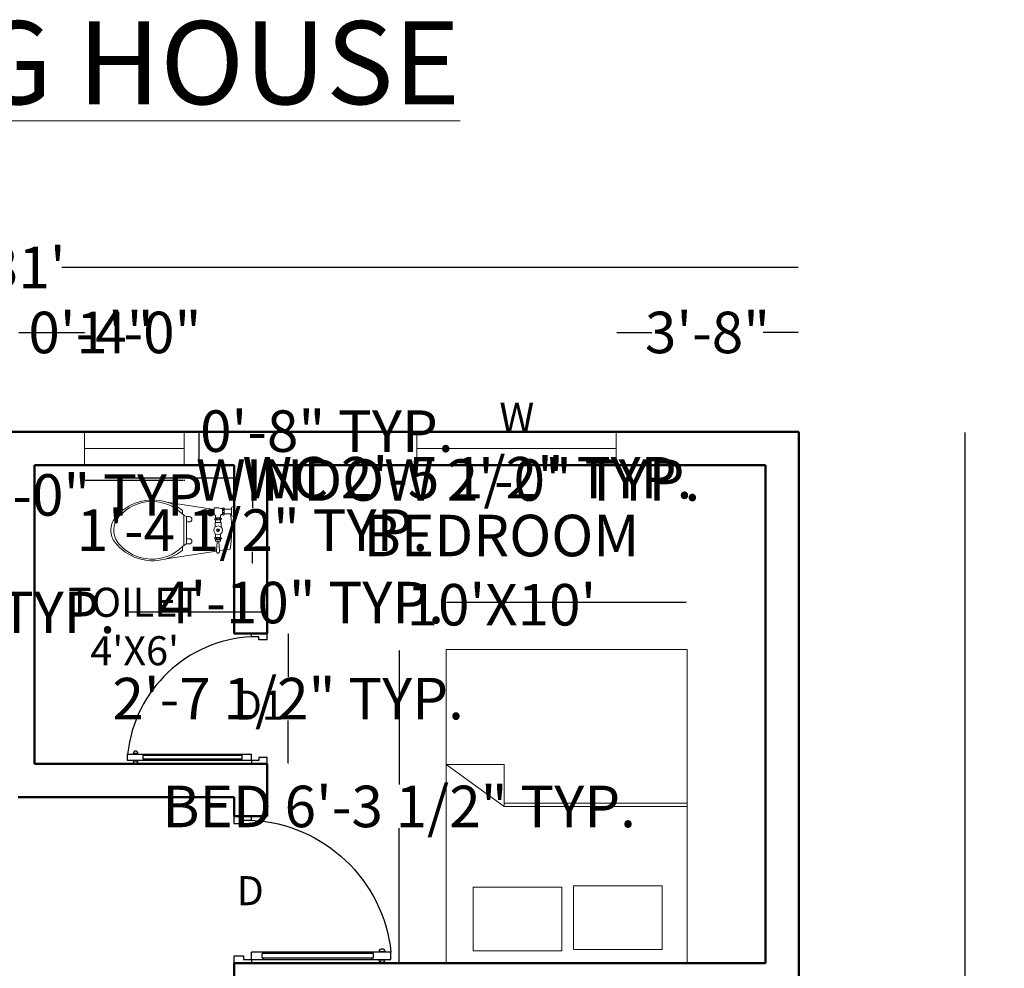
# Model space of a CAD drawing. Units: inches. Extents: x 387 to 883, y 95 to 571.
# Tile 3 of 3: x 646 to 883, y 343 to 571. Entities that reach past the tile are written whole.
import ezdxf

# ---------------------------------------------------------------- set-up
doc = ezdxf.new("R2010")
doc.units = ezdxf.units.IN
doc.header["$MEASUREMENT"] = 0
for name, color, linetype, lineweight in [('A-ANNO-DIMS', 2, 'Continuous', 18), ('A-ANNO-TEXT', 7, 'Continuous', 18), ('A-AREA-IDEN', 7, 'Continuous', 25), ('A-DOOR', 3, 'Continuous', 25), ('A-FLOR-FIXT', 8, 'Continuous', 18), ('A-FURN', 8, 'Continuous', 18), ('A-GLAZ', 4, 'Continuous', 18), ('A-WALL', 7, 'Continuous', 50)]:
    doc.layers.add(name, color=color, linetype=linetype, lineweight=lineweight)
doc.styles.get("Standard").update_dxf_attribs({"font": 'arial.ttf'})
doc.dimstyles.get("Standard").update_dxf_attribs({"dimtxt": 10, "dimasz": 0.18, "dimexe": 0.18, "dimexo": 0.0625, "dimgap": 0.09, "dimtad": 0, "dimtih": 1, "dimtoh": 1, "dimdec": 0, "dimzin": 0, "dimdsep": 46, "dimlunit": 4, "dimtxsty": 'Standard', "dimcen": 0.09, "dimse1": 1, "dimse2": 1, "dimadec": 0, "dimazin": 0, "dimtfac": 1, "dimtdec": 0, "dimtofl": 0, "dimtmove": 0, "dimatfit": 3, "dimfxl": 1, "dimtolj": 1, "dimtzin": 0, "dimarcsym": 0})

# ---------------------------------------------------------------- blocks, each defined once
blk = doc.blocks.new('w')
blk.add_line((755.51, 424.04), (707.51, 424.04))
blk.add_lwpolyline([(707.51, 420.04), (755.51, 420.04), (755.51, 428.04), (707.51, 428.04)], close=True)
blk = doc.blocks.new('w1')
for p, q in [((554.92, 428.04), (554.92, 420.04)), ((554.92, 424.04), (530.92, 424.04))]:
    blk.add_line(p, q)
blk.add_lwpolyline([(554.92, 428.04), (530.92, 428.04), (530.92, 420.04), (554.92, 420.04)])
blk = doc.blocks.new('d1')
for p, q in [((2995.74, 701.33), (2997.52, 701.33)), ((2995.74, 667.71), (2995.74, 701.33)), ((2997.52, 701.33), (2997.52, 667.71)), ((2995.6, 698.54), (2995.6, 699.83)), ((2997.66, 698.54), (2997.66, 699.83)), ((2995.74, 696.72), (2996.1, 696.72)), ((2996.1, 697.09), (2997.16, 697.09)), ((2996.1, 670.28), (2996.1, 697.09)), ((2997.16, 697.09), (2997.16, 670.28)), ((2997.16, 696.72), (2997.52, 696.72)), ((2995.74, 670.55), (2996.1, 670.55)), ((2997.16, 670.55), (2997.52, 670.55)), ((2996.1, 670.28), (2997.16, 670.28)), ((2995.74, 667.71), (2994.8, 667.71)), ((2994.8, 663.45), (2994.8, 667.71)), ((2995.74, 667.71), (2997.52, 667.71)), ((2995.74, 665.76), (2995.74, 667.71)), ((2996.58, 665.76), (2995.74, 665.76)), ((2996.58, 663.45), (2996.58, 665.76)), ((3028.53, 665.76), (3029.37, 665.76)), ((3028.53, 663.45), (3028.53, 665.76)), ((3029.37, 665.76), (3029.37, 667.71)), ((3029.37, 667.71), (3030.3, 667.71)), ((3030.3, 663.45), (3030.3, 667.71)), ((2994.8, 663.45), (2996.58, 663.45)), ((3028.53, 663.45), (3030.3, 663.45))]:
    blk.add_line(p, q)
for centre, radius, start, end in [((2993.79, 665.9), 35.62, 2.9057, 83.9884), ((2995.6, 699.19), 0.641, 90, 270), ((2997.66, 699.19), 0.641, 270, 90)]:
    blk.add_arc(centre, radius, start, end)
blk = doc.blocks.new('BED')
for p, q in [((1734.14, 2886.74), (1849.51, 2886.74)), ((1734.14, 2884.74), (1849.51, 2884.74)), ((1849.51, 2886.74), (1886.14, 2860.24)), ((1886.14, 2860.24), (1849.51, 2886.74)), ((1849.51, 2886.74), (1849.51, 2860.24)), ((1849.51, 2860.24), (1886.14, 2860.24))]:
    blk.add_line(p, q)
for points in [[(1734.14, 2787.74), (1886.14, 2787.74), (1886.14, 2985.74), (1734.14, 2985.74)], [(1749.96, 2936.84), (1805.89, 2936.84), (1805.89, 2977.01), (1749.96, 2977.01)], [(1813.22, 2937.77), (1869.15, 2937.77), (1869.15, 2977.94), (1813.22, 2977.94)]]:
    blk.add_lwpolyline(points, close=True)
blk = doc.blocks.new('TOILETY')
for p, q in [((2296.18, 1053.04), (2296.18, 1053.32)), ((2296.61, 1052.51), (2296.98, 1052.51)), ((2296.98, 1052.51), (2297.74, 1052.51)), ((2297.74, 1052.61), (2297.74, 1052.53)), ((2297.74, 1052.53), (2297.74, 1052.51)), ((2297.74, 1052.51), (2297.74, 1050.24)), ((2307.26, 1052.61), (2307.26, 1052.53)), ((2307.26, 1052.53), (2307.26, 1052.51)), ((2307.26, 1052.51), (2307.26, 1050.24)), ((2297.74, 1050.24), (2297.74, 1050.17)), ((2303.23, 1052.05), (2303.23, 1050.7)), ((2307.26, 1050.24), (2307.26, 1050.17)), ((2296.53, 1036.19), (2297.18, 1037.38)), ((2297.18, 1037.38), (2297.18, 1038.67)), ((2299.5, 1037.38), (2297.18, 1037.38)), ((2299.5, 1038.67), (2299.5, 1037.38)), ((2303.22, 1037.38), (2299.5, 1037.38)), ((2303.22, 1037.38), (2306.94, 1037.38)), ((2306.94, 1038.67), (2306.94, 1037.38)), ((2306.94, 1037.38), (2309.26, 1037.38)), ((2309.26, 1037.38), (2309.26, 1038.67)), ((2309.9, 1036.19), (2309.26, 1037.38))]:
    blk.add_line(p, q)
for points in [[(2293.85, 1057.29), (2293.28, 1057.29, -0.293225), (2292.64, 1058.42), (2294.98, 1058.42), (2297.17, 1058.42, -0.293225), (2296.54, 1057.29), (2295.97, 1057.29)], [(2294.98, 1057.29), (2293.85, 1057.29, -0.293225)], [(2294.98, 1057.29), (2295.97, 1057.29, 0.335115)], [(2295.97, 1056.9, -0.066772), (2311.57, 1056.74, -11.173493)], [(2312.2, 1051.98), (2311.57, 1056.74, 0.064477)], [(2293.85, 1054.1), (2293.63, 1054.1, 0.913215), (2293.63, 1053.32)], [(2294.91, 1054.1), (2293.85, 1054.1, 0.913215)], [(2294.91, 1054.1), (2295.97, 1054.1, -0.913215)], [(2295.97, 1054.1), (2296.18, 1054.1, -0.913215), (2296.18, 1053.32), (2296.11, 1053.32)], [(2297.78, 1052.66, 0.071269), (2297.81, 1052.53, 0.085783), (2297.9, 1052.35, 0.10607), (2298.04, 1052.23, 0.126822), (2298.2, 1052.19, 0.126822), (2298.36, 1052.23, 0.10607), (2298.5, 1052.35, 0.085783), (2298.59, 1052.53, 0.071269), (2298.62, 1052.66, 0.075445)], [(2298.66, 1052.58, 0.236068), (2298.84, 1052.47), (2299.76, 1052.47, 0.868488)], [(2306.34, 1052.58, -0.236068), (2306.17, 1052.47), (2304.79, 1052.47, -0.947474)], [(2307.23, 1052.66, -0.071269), (2307.19, 1052.53, -0.085783), (2307.1, 1052.35, -0.10607), (2306.96, 1052.23, -0.126822), (2306.8, 1052.19, -0.126822), (2306.65, 1052.23, -0.10607), (2306.5, 1052.35, -0.085783), (2306.41, 1052.53, -0.071269), (2306.38, 1052.66, -0.075445)], [(2307.26, 1052.51, 0.414214), (2307.4, 1052.44), (2307.9, 1052.47, -0.274044), (2308.04, 1052.4), (2308.04, 1051.9)], [(2290.73, 1028.75), (2293.96, 1049.64, -0.075157)], [(2297.78, 1050.12, -0.056795), (2297.81, 1050.29, -0.085783), (2297.9, 1050.46, -0.10607), (2298.04, 1050.59, -0.126822), (2298.2, 1050.63, -0.126822), (2298.36, 1050.59, -0.10607), (2298.5, 1050.46, -0.085783), (2298.59, 1050.29, -0.056795), (2298.62, 1050.12, -0.075445)], [(2298.66, 1050.17, -0.236068), (2298.84, 1050.28), (2299.76, 1050.28, -0.868488)], [(2306.34, 1050.17, 0.236068), (2306.17, 1050.28), (2304.79, 1050.28, 0.947474)], [(2307.23, 1050.12, 0.056795), (2307.19, 1050.29, 0.085783), (2307.1, 1050.46, 0.10607), (2306.96, 1050.59, 0.126822), (2306.8, 1050.63, 0.126822), (2306.65, 1050.59, 0.10607), (2306.5, 1050.46, 0.085783), (2306.41, 1050.29, 0.056795), (2306.38, 1050.12, 0.075445)], [(2307.26, 1050.24, -0.414214), (2307.4, 1050.31), (2307.9, 1050.28, 0.274044), (2308.04, 1050.35), (2308.04, 1050.84)], [(2308.04, 1051.9, 0.386607), (2308.25, 1051.76), (2312.2, 1051.98, -0.016038)], [(2308.04, 1050.84, -0.386607), (2308.25, 1050.98), (2312.4, 1050.75, 0.016063)], [(2312.2, 1051.98), (2312.68, 1052.01, -0.016603), (2312.71, 1052.01, -1.33807)], [(2312.4, 1050.75), (2312.68, 1050.74, 0.016603), (2312.71, 1050.74, 1.33807)], [(2315.84, 1028.5), (2312.4, 1050.75, 0.07524)], [(2312.71, 1052.01, -0.398884), (2313.25, 1051.55), (2313.25, 1051.37)], [(2312.71, 1050.74, 0.398884), (2313.25, 1051.2), (2313.25, 1051.37)], [(2296.03, 1035.7, 0.434217), (2297.18, 1007.59, 0.182634), (2303.22, 1005.38, 2.693815)], [(2294.42, 1035.7, 0.094048), (2290.73, 1028.75, 0.16845)], [(2296.03, 1035.7), (2294.42, 1035.7, 0.416606)], [(2296.53, 1036.19, 0.008985), (2296.03, 1035.7, 0.182634)], [(2303.22, 1036.19), (2296.53, 1036.19, 0.008985)], [(2303.22, 1036.19), (2309.9, 1036.19, -0.444938)], [(2310.4, 1035.7, -0.434217), (2309.26, 1007.59, -0.182634), (2303.22, 1005.38, -2.693815)], [(2309.9, 1036.19, -0.008985), (2310.4, 1035.7, -0.182634)], [(2310.4, 1035.7), (2312.01, 1035.7, -0.416606)], [(2312.01, 1035.7, -0.105447), (2315.97, 1027.83, -0.16845)], [(2290.73, 1028.75, 0.310397), (2297.82, 1005.91, 0.16845), (2303.22, 1004.04, 2.883082)], [(2315.97, 1027.83, -0.298065), (2308.61, 1005.91, -0.16845), (2303.22, 1004.04, -2.883082)], [(2315.97, 1027.83, 0.006132), (2315.84, 1028.5, 0.069947)]]:
    blk.add_lwpolyline(points, format="xyb")
for points in [[(2293.85, 1054.1), (2293.85, 1057.29)], [(2295.97, 1056.9), (2295.97, 1057.29)], [(2295.97, 1054.1), (2295.97, 1056.9)], [(2293.63, 1053.32), (2293.63, 1052.54), (2293.28, 1051.76), (2293.28, 1049.78)], [(2296.18, 1053.32), (2293.63, 1053.32)], [(2298.66, 1050.17), (2298.66, 1052.61)], [(2299.76, 1052.51), (2299.76, 1052.72), (2301.87, 1052.72)], [(2299.76, 1052.51), (2299.76, 1050.28)], [(2306.34, 1050.17), (2306.34, 1052.61)], [(2293.96, 1049.64), (2293.35, 1049.64), (2293.28, 1049.78)], [(2294.24, 1049.64), (2293.96, 1049.64)], [(2294.17, 1049.46), (2294.24, 1049.46)], [(2294.34, 1048.89), (2294.17, 1048.89), (2294.17, 1049.46)], [(2294.17, 1049.46), (2294.45, 1049.38), (2294.81, 1049.46), (2295.16, 1049.38), (2295.44, 1049.46)], [(2294.17, 1048.89), (2294.45, 1048.96), (2294.81, 1048.89), (2295.16, 1048.96), (2295.44, 1048.89)], [(2294.24, 1049.46), (2294.24, 1049.64)], [(2295.37, 1049.64), (2294.24, 1049.64)], [(2294.24, 1049.46), (2295.37, 1049.46)], [(2294.34, 1048.89), (2294.34, 1048.51), (2294.58, 1048.51)], [(2295.26, 1048.89), (2294.34, 1048.89)], [(2294.45, 1048.96), (2294.45, 1049.38)], [(2294.58, 1048.51), (2295.26, 1048.51), (2295.26, 1048.89)], [(2295.16, 1048.96), (2295.16, 1049.38)], [(2295.37, 1049.46), (2295.44, 1049.46), (2295.44, 1048.89), (2295.26, 1048.89)], [(2296.32, 1049.78), (2296.25, 1049.64), (2295.37, 1049.64)], [(2295.37, 1049.46), (2295.37, 1049.64)], [(2296.33, 1049.78), (2296.56, 1050.24)], [(2296.56, 1050.24), (2297.74, 1050.24)], [(2299.76, 1050.28), (2299.76, 1050.06), (2301.84, 1050.06)], [(2308.04, 1051.9), (2308.04, 1051.37)], [(2308.04, 1050.84), (2308.04, 1051.37)]]:
    blk.add_lwpolyline(points)
for points in [[(2294.91, 1053.32, 0.06206), (2295.16, 1053.35, 0.075298), (2295.36, 1053.43, 0.107049), (2295.5, 1053.57, 0.150029), (2295.55, 1053.71, 0.150029), (2295.5, 1053.85, 0.107049), (2295.36, 1053.99, 0.075298), (2295.16, 1054.07, 0.06206), (2294.91, 1054.1, 0.06206), (2294.65, 1054.07, 0.075298), (2294.46, 1053.99, 0.107049), (2294.31, 1053.85, 0.150029), (2294.27, 1053.71, 0.150029), (2294.31, 1053.57, 0.107049), (2294.46, 1053.43, 0.075298), (2294.65, 1053.35, 0.06206)], [(2298.63, 1051.37, -0.075445), (2298.59, 1051.15, -0.085783), (2298.5, 1050.97, -0.10607), (2298.36, 1050.85, -0.126822), (2298.2, 1050.81, -0.126822), (2298.04, 1050.85, -0.10607), (2297.9, 1050.97, -0.085783), (2297.81, 1051.15, -0.075445), (2297.78, 1051.37, -0.075445), (2297.81, 1051.6, -0.085783), (2297.9, 1051.77, -0.10607), (2298.04, 1051.9, -0.126822), (2298.2, 1051.94, -0.126822), (2298.36, 1051.9, -0.10607), (2298.5, 1051.77, -0.085783), (2298.59, 1051.6, -0.075445)], [(2306.38, 1051.37, 0.075445), (2306.41, 1051.15, 0.085783), (2306.5, 1050.97, 0.10607), (2306.65, 1050.85, 0.126822), (2306.8, 1050.81, 0.126822), (2306.96, 1050.85, 0.10607), (2307.1, 1050.97, 0.085783), (2307.19, 1051.15, 0.075445), (2307.23, 1051.37, 0.075445), (2307.19, 1051.6, 0.085783), (2307.1, 1051.77, 0.10607), (2306.96, 1051.9, 0.126822), (2306.8, 1051.94, 0.126822), (2306.65, 1051.9, 0.10607), (2306.5, 1051.77, 0.085783), (2306.41, 1051.6, 0.075445)]]:
    blk.add_lwpolyline(points, format="xyb", close=True)
blk.add_lwpolyline([(2303.23, 1052.05), (2302.65, 1051.71), (2302.65, 1051.04), (2303.23, 1050.7), (2303.81, 1051.04), (2303.81, 1051.71)], close=True)
blk.add_circle((2303.23, 1051.37), 1.91)
for centre, radius, start, end in [((2293.74, 1053.71), 0.391, 275.1944, 84.8056), ((2296.08, 1053.71), 0.391, 95.1944, 264.8056), ((2296.71, 1053.02), 0.527, 178.4608, 258.8588), ((2298.2, 1052.31), 0.551, 33.3985, 146.6015), ((2306.8, 1052.31), 0.551, 33.3985, 146.6015), ((2298.2, 1050.47), 0.551, 213.3985, 326.6015), ((2306.8, 1050.47), 0.551, 213.3985, 326.6015), ((2298.34, 1038.67), 1.16, 0, 180), ((2308.1, 1038.67), 1.16, 0, 180)]:
    blk.add_arc(centre, radius, start, end)
blk = doc.blocks.new('*D11')
at = {"layer": 'A-ANNO-DIMS', "color": 0, "lineweight": -2, "transparency": 16777216}
for p, q in [((462.03, 511.61), (639.28, 511.61)), ((833.67, 511.61), (656.42, 511.61))]:
    blk.add_line(p, q, dxfattribs=at)
at = {"layer": 'A-ANNO-DIMS', "color": 0, "transparency": 16777216}
for points in [[(462.03, 511.64), (462.03, 511.58), (461.85, 511.61)], [(833.67, 511.64), (833.67, 511.58), (833.85, 511.61)]]:
    blk.add_solid(points, dxfattribs=at)
at = {"layer": 'Defpoints', "color": 0, "transparency": 16777216}
for p in [(461.85, 511.61), (461.85, 472), (833.85, 472)]:
    blk.add_point(p, dxfattribs=at)
at = {"layer": 'A-ANNO-DIMS', "color": 0, "transparency": 16777216, "insert": (647.85, 511.61), "char_height": 10, "attachment_point": 5}
blk.add_mtext("\\A1;31'", dxfattribs=at)
blk = doc.blocks.new('*D12')
at = {"layer": 'A-ANNO-DIMS', "color": 0, "lineweight": -2, "transparency": 16777216}
for p, q in [((873.84, 471.82), (873.84, 327.19)), ((873.84, 172.18), (873.84, 316.8))]:
    blk.add_line(p, q, dxfattribs=at)
at = {"layer": 'A-ANNO-DIMS', "color": 0, "transparency": 16777216}
for points in [[(873.81, 471.82), (873.87, 471.82), (873.84, 472)], [(873.81, 172.18), (873.87, 172.18), (873.84, 172)]]:
    blk.add_solid(points, dxfattribs=at)
at = {"layer": 'Defpoints', "color": 0, "transparency": 16777216}
for p in [(833.85, 472), (833.85, 172), (873.84, 172)]:
    blk.add_point(p, dxfattribs=at)
at = {"layer": 'A-ANNO-DIMS', "color": 0, "transparency": 16777216, "insert": (873.84, 322), "char_height": 10, "attachment_point": 5}
blk.add_mtext("\\A1;25'", dxfattribs=at)
blk = doc.blocks.new('*D13')
at = {"layer": 'A-ANNO-DIMS', "color": 0, "lineweight": -2, "transparency": 16777216}
for p, q in [((506.03, 456.8), (553.67, 456.8)), ((553.85, 456.8), (554.03, 456.8))]:
    blk.add_line(p, q, dxfattribs=at)
at = {"layer": 'A-ANNO-DIMS', "color": 0, "transparency": 16777216}
for points in [[(506.03, 456.83), (506.03, 456.77), (505.85, 456.8)], [(553.67, 456.83), (553.67, 456.77), (553.85, 456.8)]]:
    blk.add_solid(points, dxfattribs=at)
at = {"layer": 'Defpoints', "color": 0, "transparency": 16777216}
for p in [(505.85, 464), (553.85, 464), (553.85, 456.8)]:
    blk.add_point(p, dxfattribs=at)
at = {"layer": 'A-ANNO-DIMS', "color": 0, "transparency": 16777216, "insert": (625.93, 456.8), "char_height": 10, "attachment_point": 5}
blk.add_mtext('\\A1;WINDOW W 4\'-0" TYP.', dxfattribs=at)
blk = doc.blocks.new('*D15')
at = {"layer": 'A-ANNO-DIMS', "color": 0, "lineweight": -2, "transparency": 16777216}
for p, q in [((662.03, 460.4), (685.67, 460.4)), ((685.85, 460.4), (686.03, 460.4))]:
    blk.add_line(p, q, dxfattribs=at)
at = {"layer": 'A-ANNO-DIMS', "color": 0, "transparency": 16777216}
for points in [[(662.03, 460.43), (662.03, 460.37), (661.85, 460.4)], [(685.67, 460.43), (685.67, 460.37), (685.85, 460.4)]]:
    blk.add_solid(points, dxfattribs=at)
at = {"layer": 'Defpoints', "color": 0, "transparency": 16777216}
for p in [(661.85, 464), (685.85, 464), (685.85, 460.4)]:
    blk.add_point(p, dxfattribs=at)
at = {"layer": 'A-ANNO-DIMS', "color": 0, "transparency": 16777216, "insert": (749.39, 460.4), "char_height": 10, "attachment_point": 5}
blk.add_mtext('\\A1;WINDOW 2\'-0" TYP.', dxfattribs=at)
blk = doc.blocks.new('*D16')
at = {"layer": 'A-ANNO-DIMS', "color": 0, "lineweight": -2, "transparency": 16777216}
for p, q in [((689.45, 472), (689.45, 472.18)), ((689.45, 472.18), (689.63, 472.18)), ((689.45, 464.18), (689.45, 471.82))]:
    blk.add_line(p, q, dxfattribs=at)
at = {"layer": 'A-ANNO-DIMS', "color": 0, "transparency": 16777216}
for points in [[(689.42, 471.82), (689.48, 471.82), (689.45, 472)], [(689.42, 464.18), (689.48, 464.18), (689.45, 464)]]:
    blk.add_solid(points, dxfattribs=at)
at = {"layer": 'Defpoints', "color": 0, "transparency": 16777216}
for p in [(685.85, 472), (689.45, 472), (685.85, 464)]:
    blk.add_point(p, dxfattribs=at)
at = {"layer": 'A-ANNO-DIMS', "color": 0, "transparency": 16777216, "insert": (720.2, 472.18), "char_height": 10, "attachment_point": 5}
blk.add_mtext('\\A1;0\'-8" TYP.', dxfattribs=at)
blk = doc.blocks.new('*D17')
at = {"layer": 'A-ANNO-DIMS', "color": 0, "lineweight": -2, "transparency": 16777216}
for p, q in [((672.24, 428.54), (672.06, 428.54)), ((705.67, 428.54), (672.42, 428.54))]:
    blk.add_line(p, q, dxfattribs=at)
at = {"layer": 'A-ANNO-DIMS', "color": 0, "transparency": 16777216}
for points in [[(672.42, 428.57), (672.42, 428.51), (672.24, 428.54)], [(705.67, 428.57), (705.67, 428.51), (705.85, 428.54)]]:
    blk.add_solid(points, dxfattribs=at)
at = {"layer": 'Defpoints', "color": 0, "transparency": 16777216}
for p in [(672.24, 428.54), (672.24, 423.5), (705.85, 423.5)]:
    blk.add_point(p, dxfattribs=at)
at = {"layer": 'A-ANNO-DIMS', "color": 0, "transparency": 16777216, "insert": (596.32, 428.54), "char_height": 10, "attachment_point": 5}
blk.add_mtext('\\A1;DOOR D1 2\'-9 1/2" TYP.', dxfattribs=at)
blk = doc.blocks.new('*D18')
at = {"layer": 'A-ANNO-DIMS', "color": 0, "lineweight": -2, "transparency": 16777216}
for p, q in [((710.89, 423.32), (710.89, 413.01)), ((710.89, 392.18), (710.89, 402.49))]:
    blk.add_line(p, q, dxfattribs=at)
at = {"layer": 'A-ANNO-DIMS', "color": 0, "transparency": 16777216}
for points in [[(710.86, 423.32), (710.92, 423.32), (710.89, 423.5)], [(710.86, 392.18), (710.92, 392.18), (710.89, 392)]]:
    blk.add_solid(points, dxfattribs=at)
at = {"layer": 'Defpoints', "color": 0, "transparency": 16777216}
for p in [(705.85, 423.5), (710.89, 423.5), (705.85, 392)]:
    blk.add_point(p, dxfattribs=at)
at = {"layer": 'A-ANNO-DIMS', "color": 0, "transparency": 16777216, "insert": (710.89, 407.75), "char_height": 10, "attachment_point": 5}
blk.add_mtext('\\A1;2\'-7 1/2" TYP.', dxfattribs=at)
blk = doc.blocks.new('*D21')
at = {"layer": 'A-ANNO-DIMS', "color": 0, "lineweight": -2, "transparency": 16777216}
for p, q in [((737.6, 419.37), (737.6, 387.04)), ((737.6, 344.18), (737.6, 376.51))]:
    blk.add_line(p, q, dxfattribs=at)
at = {"layer": 'A-ANNO-DIMS', "color": 0, "transparency": 16777216}
for points in [[(737.57, 419.37), (737.63, 419.37), (737.6, 419.55)], [(737.57, 344.18), (737.63, 344.18), (737.6, 344)]]:
    blk.add_solid(points, dxfattribs=at)
at = {"layer": 'Defpoints', "color": 0, "transparency": 16777216}
for p in [(748.93, 419.55), (737.6, 344), (748.93, 344)]:
    blk.add_point(p, dxfattribs=at)
at = {"layer": 'A-ANNO-DIMS', "color": 0, "transparency": 16777216, "insert": (737.6, 381.77), "char_height": 10, "attachment_point": 5}
blk.add_mtext('\\A1;BED 6\'-3 1/2" TYP.', dxfattribs=at)
blk = doc.blocks.new('*D22')
at = {"layer": 'A-ANNO-DIMS', "color": 0, "lineweight": -2, "transparency": 16777216}
for p, q in [((748.93, 430.88), (748.75, 430.88)), ((806.75, 430.88), (749.11, 430.88))]:
    blk.add_line(p, q, dxfattribs=at)
at = {"layer": 'A-ANNO-DIMS', "color": 0, "transparency": 16777216}
for points in [[(749.11, 430.91), (749.11, 430.85), (748.93, 430.88)], [(806.75, 430.91), (806.75, 430.85), (806.93, 430.88)]]:
    blk.add_solid(points, dxfattribs=at)
at = {"layer": 'Defpoints', "color": 0, "transparency": 16777216}
for p in [(748.93, 430.88), (748.93, 419.55), (806.93, 419.55)]:
    blk.add_point(p, dxfattribs=at)
at = {"layer": 'A-ANNO-DIMS', "color": 0, "transparency": 16777216, "insert": (714.1, 430.88), "char_height": 10, "attachment_point": 5}
blk.add_mtext('\\A1;4\'-10" TYP.', dxfattribs=at)
blk = doc.blocks.new('*D23')
at = {"layer": 'A-ANNO-DIMS', "color": 0, "lineweight": -2, "transparency": 16777216}
for p, q in [((668.38, 460.95), (697.67, 460.95)), ((697.85, 460.95), (698.03, 460.95))]:
    blk.add_line(p, q, dxfattribs=at)
at = {"layer": 'A-ANNO-DIMS', "color": 0, "transparency": 16777216}
for points in [[(668.38, 460.98), (668.38, 460.92), (668.2, 460.95)], [(697.67, 460.98), (697.67, 460.92), (697.85, 460.95)]]:
    blk.add_solid(points, dxfattribs=at)
at = {"layer": 'Defpoints', "color": 0, "transparency": 16777216}
for p in [(697.85, 460.95), (668.2, 456.51), (697.85, 456.51)]:
    blk.add_point(p, dxfattribs=at)
at = {"layer": 'A-ANNO-DIMS', "color": 0, "transparency": 16777216, "insert": (754.03, 460.95), "char_height": 10, "attachment_point": 5}
blk.add_mtext('\\A1;WC 2\'-5 1/2" TYP.', dxfattribs=at)
blk = doc.blocks.new('*D24')
at = {"layer": 'A-ANNO-DIMS', "color": 0, "lineweight": -2, "transparency": 16777216}
for p, q in [((702.3, 456.33), (702.3, 453.6)), ((702.3, 440.36), (702.3, 443.08))]:
    blk.add_line(p, q, dxfattribs=at)
at = {"layer": 'A-ANNO-DIMS', "color": 0, "transparency": 16777216}
for points in [[(702.27, 456.33), (702.33, 456.33), (702.3, 456.51)], [(702.27, 440.36), (702.33, 440.36), (702.3, 440.18)]]:
    blk.add_solid(points, dxfattribs=at)
at = {"layer": 'Defpoints', "color": 0, "transparency": 16777216}
for p in [(697.85, 456.51), (697.85, 440.18), (702.3, 440.18)]:
    blk.add_point(p, dxfattribs=at)
at = {"layer": 'A-ANNO-DIMS', "color": 0, "transparency": 16777216, "insert": (702.3, 448.34), "char_height": 10, "attachment_point": 5}
blk.add_mtext('\\A1;1\'-4 1/2" TYP.', dxfattribs=at)
blk = doc.blocks.new('*D34')
at = {"layer": 'A-ANNO-DIMS', "color": 0, "lineweight": -2, "transparency": 16777216}
for p, q in [((790.03, 495.95), (798.47, 495.95)), ((833.67, 495.95), (825.23, 495.95))]:
    blk.add_line(p, q, dxfattribs=at)
at = {"layer": 'A-ANNO-DIMS', "color": 0, "transparency": 16777216}
for points in [[(790.03, 495.98), (790.03, 495.92), (789.85, 495.95)], [(833.67, 495.98), (833.67, 495.92), (833.85, 495.95)]]:
    blk.add_solid(points, dxfattribs=at)
at = {"layer": 'Defpoints', "color": 0, "transparency": 16777216}
for p in [(789.85, 495.95), (789.85, 472), (833.85, 472)]:
    blk.add_point(p, dxfattribs=at)
at = {"layer": 'A-ANNO-DIMS', "color": 0, "transparency": 16777216, "insert": (811.85, 495.95), "char_height": 10, "attachment_point": 5}
blk.add_mtext('\\A1;3\'-8"', dxfattribs=at)
blk = doc.blocks.new('*D40')
at = {"layer": 'A-ANNO-DIMS', "color": 0, "lineweight": -2, "transparency": 16777216}
for p, q in [((650.03, 495.95), (661.67, 495.95)), ((661.85, 495.95), (662.03, 495.95))]:
    blk.add_line(p, q, dxfattribs=at)
at = {"layer": 'A-ANNO-DIMS', "color": 0, "transparency": 16777216}
for points in [[(650.03, 495.98), (650.03, 495.92), (649.85, 495.95)], [(661.67, 495.98), (661.67, 495.92), (661.85, 495.95)]]:
    blk.add_solid(points, dxfattribs=at)
at = {"layer": 'Defpoints', "color": 0, "transparency": 16777216}
for p in [(661.85, 495.95), (649.85, 464), (661.85, 464)]:
    blk.add_point(p, dxfattribs=at)
at = {"layer": 'A-ANNO-DIMS', "color": 0, "transparency": 16777216, "insert": (674.94, 495.95), "char_height": 10, "attachment_point": 5}
blk.add_mtext('\\A1;1\'-0"', dxfattribs=at)
blk = doc.blocks.new('*D41')
at = {"layer": 'A-ANNO-DIMS', "color": 0, "lineweight": -2, "transparency": 16777216}
for p, q in [((646.03, 495.95), (649.67, 495.95)), ((649.85, 495.95), (650.03, 495.95))]:
    blk.add_line(p, q, dxfattribs=at)
at = {"layer": 'A-ANNO-DIMS', "color": 0, "transparency": 16777216}
for points in [[(646.03, 495.98), (646.03, 495.92), (645.85, 495.95)], [(649.67, 495.98), (649.67, 495.92), (649.85, 495.95)]]:
    blk.add_solid(points, dxfattribs=at)
at = {"layer": 'Defpoints', "color": 0, "transparency": 16777216}
for p in [(649.85, 495.95), (645.85, 464), (649.85, 464)]:
    blk.add_point(p, dxfattribs=at)
at = {"layer": 'A-ANNO-DIMS', "color": 0, "transparency": 16777216, "insert": (663.41, 495.95), "char_height": 10, "attachment_point": 5}
blk.add_mtext('\\A1;0\'-4"', dxfattribs=at)
blk = doc.blocks.new('*D44')
at = {"layer": 'A-ANNO-DIMS', "color": 0, "lineweight": -2, "transparency": 16777216}
for p, q in [((437.9, 463.82), (437.9, 461.41)), ((437.9, 448.47), (437.9, 450.88))]:
    blk.add_line(p, q, dxfattribs=at)
at = {"layer": 'A-ANNO-DIMS', "color": 0, "transparency": 16777216}
for points in [[(437.87, 463.82), (437.93, 463.82), (437.9, 464)], [(437.87, 448.47), (437.93, 448.47), (437.9, 448.29)]]:
    blk.add_solid(points, dxfattribs=at)
at = {"layer": 'Defpoints', "color": 0, "transparency": 16777216}
for p in [(649.85, 464), (437.9, 448.29), (668.2, 448.29)]:
    blk.add_point(p, dxfattribs=at)
at = {"layer": 'A-ANNO-DIMS', "color": 0, "transparency": 16777216, "insert": (437.9, 456.14), "char_height": 10, "attachment_point": 5}
blk.add_mtext('\\A1;1\'-3 1/2"', dxfattribs=at)

msp = doc.modelspace()

# ---------------------------------------------------------------- linework, layer by layer
at = {"layer": 'A-WALL'}
for p, q in [((461.85, 472), (833.85, 472)), ((833.85, 172), (833.85, 472)), ((649.85, 464), (697.85, 464)), ((649.85, 392), (649.85, 464)), ((697.85, 423.4), (697.85, 464)), ((705.85, 464), (825.85, 464)), ((705.85, 423.4), (705.85, 464)), ((825.85, 344), (825.85, 464)), ((697.85, 423.4), (705.85, 423.4)), ((649.85, 392), (705.85, 392)), ((705.85, 379.4), (705.85, 392)), ((645.85, 384), (697.85, 384)), ((697.85, 379.4), (697.85, 384)), ((697.85, 379.4), (705.85, 379.4)), ((697.85, 344), (825.85, 344)), ((697.85, 336), (697.85, 344))]:
    msp.add_line(p, q, dxfattribs=at)

# ---------------------------------------------------------------- block references
at = {"layer": 'A-DOOR'}
for p, xscale, yscale, zscale, rotation in [((1294.55, -2265.37), 0.8873243955715187, 0.8873243955715187, 0.8873243955715187, 90), ((36.27, -2642.37), -0.9971830985915492, 0.9971830985915492, 0.9971830985915492, 270)]:
    msp.add_blockref('d1', p, dxfattribs=dict(at, xscale=xscale, yscale=yscale, zscale=zscale, rotation=rotation))
at = {"layer": 'A-FLOR-FIXT', "xscale": 0.5452019050314921, "yscale": 0.5452019050314921, "zscale": 0.5452019050314921, "rotation": 270}
msp.add_blockref('TOILETY', (120.8, 1704.01), dxfattribs=at)
at = {"layer": 'A-FURN', "xscale": 0.381578947368421, "yscale": 0.381578947368421, "zscale": 0.381578947368421, "rotation": 180}
msp.add_blockref('BED', (1468.65, 1483.29), dxfattribs=at)
at = {"layer": 'A-GLAZ'}
for name, p in [('w1', (130.93, 43.96)), ('w', (34.34, 43.96))]:
    msp.add_blockref(name, p, dxfattribs=at)

# ---------------------------------------------------------------- texts
at = {"layer": 'A-ANNO-TEXT', "attachment_point": 1}
for s, width, insert, char_height in [('{\\fArial|b1|i0|c0|p34;\\LEAST FACING HOUSE\\l }', 366.1947, (487.14, 570.93), 20), ('\\pxqc;W', 47.8337, (742.02, 479), 7), ('\\pxqc;D1', 47.8337, (680.02, 409.67), 7), ('\\pxqc;D', 47.8337, (677.84, 364.98), 7)]:
    msp.add_mtext_dynamic_manual_height_columns(s, width=width, gutter_width=1, heights=[0], dxfattribs=dict(at, insert=insert, char_height=char_height))
at = {"layer": 'A-AREA-IDEN', "attachment_point": 1}
for s, insert, char_height in [("\\pxqc;BEDROOM\\P10'X10'", (738.33, 452.03), 10), ("\\pxqc;TOILET\\P4'X6'", (650.02, 434.45), 7)]:
    msp.add_mtext_dynamic_manual_height_columns(s, width=47.8337, gutter_width=1, heights=[0], dxfattribs=dict(at, insert=insert, char_height=char_height))

# ---------------------------------------------------------------- dimensions: what is measured, and where the dimension line sits
at = {"layer": 'A-ANNO-DIMS'}
for p2, distance, picture, middle in [((461.85, 472), -39.61, '*D11', (647.85, 511.61)), ((833.85, 172), 39.99, '*D12', (873.84, 322))]:
    dim = msp.add_aligned_dim(p1=(833.85, 472), p2=p2, distance=distance, dimstyle='Standard', override={"dimclrd": 0, "dimclre": 0, "dimclrt": 0}, dxfattribs=at)
    dim.commit()
    dim.dimension.update_dxf_attribs({"geometry": picture, "text_midpoint": middle})
for base, p1, p2, picture, middle in [((649.85, 495.95), (645.85, 464), (649.85, 464), '*D41', (663.41, 495.95)), ((661.85, 495.95), (649.85, 464), (661.85, 464), '*D40', (674.94, 495.95)), ((789.85, 495.95), (833.85, 472), (789.85, 472), '*D34', (811.85, 495.95))]:
    dim = msp.add_linear_dim(base=base, p1=p1, p2=p2, dimstyle='Standard', override={"dimdec": 1, "dimlfac": 1, "dimrnd": 0, "dimzin": 1, "dimdsep": 46, "dimlunit": 4, "dimfrac": 2}, dxfattribs=at)
    dim.commit()
    dim.dimension.update_dxf_attribs({"geometry": picture, "text_midpoint": middle})
for base, p1, p2, text, picture, middle in [((697.8516, 460.9545), (668.2048, 456.5074), (697.8516, 456.5074), 'WC <> TYP.', '*D23', (754.0323, 460.9545)), ((553.85, 456.8), (505.85, 464), (553.85, 464), 'WINDOW W <> TYP.', '*D13', (625.93, 456.8)), ((685.85, 460.4), (661.85, 464), (685.85, 464), 'WINDOW <> TYP.', '*D15', (749.39, 460.4))]:
    dim = msp.add_linear_dim(base=base, p1=p1, p2=p2, text=text, dimstyle='Standard', override={"dimdec": 1, "dimlfac": 1, "dimrnd": 0, "dimzin": 1, "dimdsep": 46, "dimlunit": 4, "dimfrac": 2}, dxfattribs=at)
    dim.commit()
    dim.dimension.update_dxf_attribs({"geometry": picture, "text_midpoint": middle})
for base, p1, p2, angle, text, picture, middle in [((689.45, 472), (685.85, 464), (685.85, 472), 90, '<> TYP.', '*D16', (720.2, 472.18)), ((702.3, 440.18), (697.85, 456.51), (697.85, 440.18), 270, '<> TYP.', '*D24', (702.3, 448.34)), ((672.24, 428.54), (705.85, 423.5), (672.24, 423.5), 180, 'DOOR D1 <> TYP.', '*D17', (596.32, 428.54)), ((748.93, 430.88), (806.93, 419.55), (748.93, 419.55), 180, '<> TYP.', '*D22', (714.1, 430.88)), ((710.89, 423.5), (705.85, 392), (705.85, 423.5), 90, '<> TYP.', '*D18', (710.89, 407.75)), ((737.6018, 343.9978), (748.9347, 419.5504), (748.9347, 343.9978), 270, 'BED <> TYP.', '*D21', (737.6018, 381.7741))]:
    dim = msp.add_linear_dim(base=base, p1=p1, p2=p2, angle=angle, text=text, dimstyle='Standard', override={"dimdec": 1, "dimlfac": 1, "dimrnd": 0, "dimzin": 1, "dimdsep": 46, "dimlunit": 4, "dimfrac": 2}, dxfattribs=at)
    dim.commit()
    dim.dimension.update_dxf_attribs({"geometry": picture, "text_midpoint": middle})
dim = msp.add_linear_dim(base=(437.9, 448.29), p1=(649.85, 464), p2=(668.2, 448.29), angle=90, dimstyle='Standard', override={"dimdec": 1, "dimlfac": 1, "dimrnd": 0, "dimzin": 1, "dimdsep": 46, "dimlunit": 4, "dimfrac": 2}, dxfattribs=at)
dim.commit()
dim.dimension.update_dxf_attribs({"geometry": '*D44', "text_midpoint": (437.9, 456.14)})

doc.saveas('drawing.dxf')
